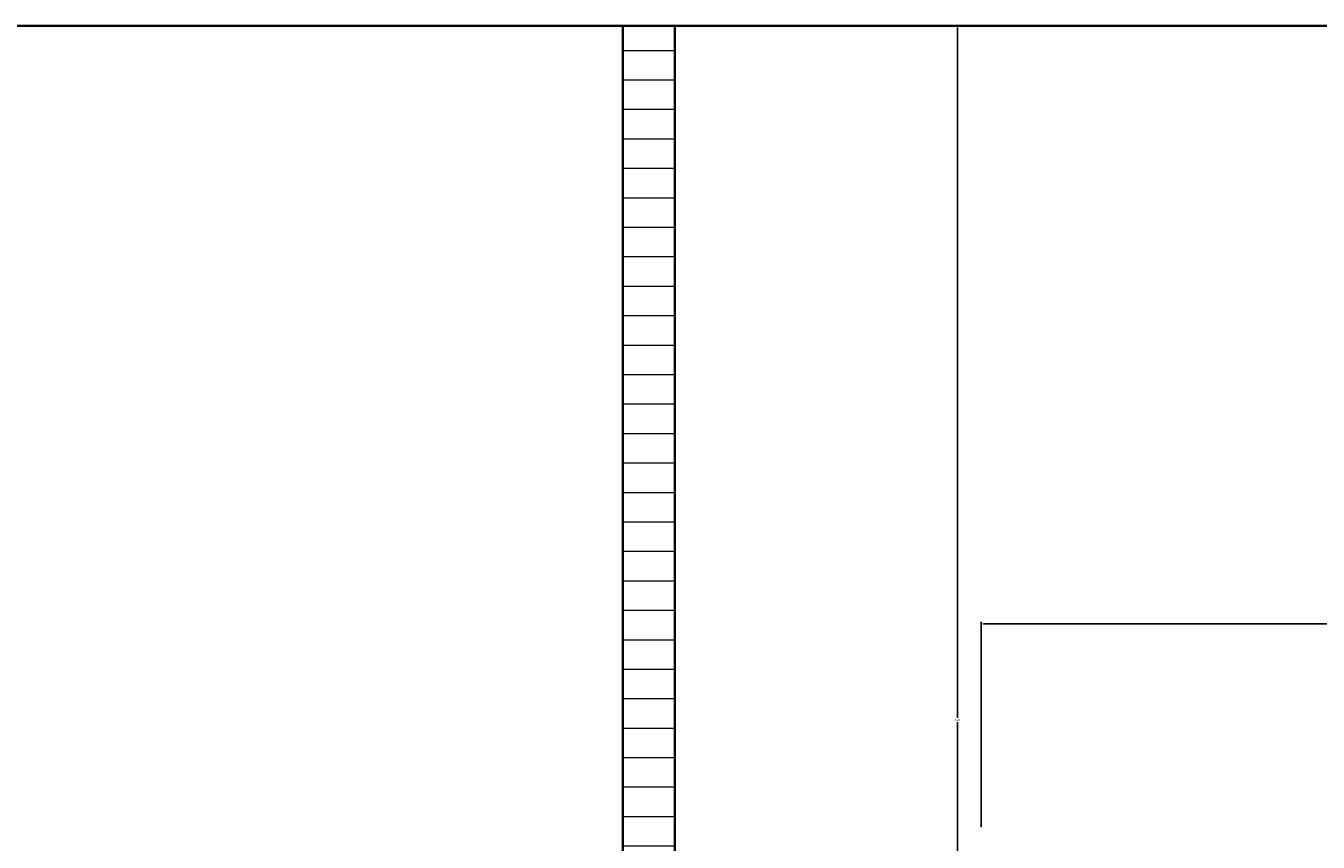
# Model space of a CAD drawing. Units: inches. Extents: x 2416 to 3391, y 1375 to 2496.
# Tile 10 of 13: x 2994 to 3105, y 2193 to 2264. Entities that reach past the tile are written whole.
import ezdxf

# ---------------------------------------------------------------- set-up
doc = ezdxf.new("R2010")
doc.units = ezdxf.units.IN
for name, color, linetype, lineweight in [('A-ANNO-DIMS', 2, 'Continuous', 18), ('A-SECT', 7, 'Continuous', 35), ('A-WALL-PATT', 252, 'Continuous', 13)]:
    doc.layers.add(name, color=color, linetype=linetype, lineweight=lineweight)
doc.styles.get("Standard").update_dxf_attribs({"font": 'arial.ttf'})
doc.dimstyles.get("Standard").update_dxf_attribs({"dimtxt": 0.18, "dimasz": 0.18, "dimexe": 0.18, "dimexo": 0.0625, "dimgap": 0.09, "dimtad": 0, "dimtih": 1, "dimtoh": 1, "dimdec": 4, "dimzin": 0, "dimdsep": 46, "dimtxsty": 'Standard', "dimcen": 0.09, "dimadec": 0, "dimazin": 0, "dimtfac": 1, "dimtdec": 4, "dimtofl": 0, "dimtmove": 0, "dimatfit": 3, "dimfxl": 1, "dimtolj": 1, "dimtzin": 0, "dimarcsym": 0})

# ---------------------------------------------------------------- blocks, each defined once
blk = doc.blocks.new('*D45')
at = {"layer": 'A-ANNO-DIMS', "color": 0, "lineweight": -2, "transparency": 16777216}
for p, q in [((3076.16, 2194.58), (3076.16, 2212.34)), ((3076.34, 2212.16), (3133.82, 2212.16)), ((3193.6, 2212.16), (3136.12, 2212.16)), ((3193.78, 2194.58), (3193.78, 2212.34))]:
    blk.add_line(p, q, dxfattribs=at)
at = {"layer": 'A-ANNO-DIMS', "color": 0, "transparency": 16777216}
for points in [[(3076.34, 2212.19), (3076.34, 2212.13), (3076.16, 2212.16)], [(3193.6, 2212.19), (3193.6, 2212.13), (3193.78, 2212.16)]]:
    blk.add_solid(points, dxfattribs=at)
at = {"layer": 'Defpoints', "color": 0, "transparency": 16777216}
for p in [(3076.16, 2212.16), (3076.16, 2194.51), (3193.78, 2194.51)]:
    blk.add_point(p, dxfattribs=at)
at = {"layer": 'A-ANNO-DIMS', "color": 0, "transparency": 16777216, "insert": (3134.97, 2212.16), "char_height": 0.18, "attachment_point": 5}
blk.add_mtext('\\A1;BED PROFILE 118', dxfattribs=at)
blk = doc.blocks.new('*D86')
at = {"layer": 'A-ANNO-DIMS', "color": 0, "lineweight": -2, "transparency": 16777216}
for p, q in [((3049.75, 2263.86), (3074.27, 2263.86)), ((3074.09, 2263.68), (3074.09, 2204.04)), ((3074.09, 2144.04), (3074.09, 2203.68)), ((3049.75, 2143.86), (3074.27, 2143.86))]:
    blk.add_line(p, q, dxfattribs=at)
at = {"layer": 'A-ANNO-DIMS', "color": 0, "transparency": 16777216}
for points in [[(3074.06, 2263.68), (3074.12, 2263.68), (3074.09, 2263.86)], [(3074.06, 2144.04), (3074.12, 2144.04), (3074.09, 2143.86)]]:
    blk.add_solid(points, dxfattribs=at)
at = {"layer": 'Defpoints', "color": 0, "transparency": 16777216}
for p in [(3049.69, 2263.86), (3049.69, 2143.86), (3074.09, 2143.86)]:
    blk.add_point(p, dxfattribs=at)
at = {"layer": 'A-ANNO-DIMS', "color": 0, "transparency": 16777216, "insert": (3074.09, 2203.86), "char_height": 0.18, "attachment_point": 5}
blk.add_mtext('\\A1;120', dxfattribs=at)

msp = doc.modelspace()

# ---------------------------------------------------------------- hatches: boundary and pattern name
at = {"layer": 'A-WALL-PATT'}
h = msp.add_hatch(dxfattribs=at)
h.set_pattern_fill('ANSI31', color=256, scale=0.802205, angle=-45, style=0)
h.paths.add_polyline_path([(3045.1924, 2143.8608), (3049.6924, 2143.8608), (3049.6924, 2263.8608), (3045.1924, 2263.8608)])

# ---------------------------------------------------------------- linework, layer by layer
at = {"layer": 'A-SECT'}
for p, q in [((3202.6924, 2263.8608), (2904.1924, 2263.8608)), ((3045.1924, 2263.8608), (3045.1924, 2143.8608)), ((3049.6924, 2263.8608), (3049.6924, 2143.8608))]:
    msp.add_line(p, q, dxfattribs=at)

# ---------------------------------------------------------------- dimensions: what is measured, and where the dimension line sits
at = {"layer": 'A-ANNO-DIMS'}
dim = msp.add_linear_dim(base=(3074.0924, 2143.8608), p1=(3049.6924, 2263.8608), p2=(3049.6924, 2143.8608), angle=270, dimstyle='Standard', override={"dimdec": 0, "dimlfac": 1, "dimrnd": 0, "dimzin": 0, "dimdsep": 46, "dimlunit": 2}, dxfattribs=at)
dim.commit()
dim.dimension.update_dxf_attribs({"geometry": '*D86', "text_midpoint": (3074.0924, 2203.8608)})
dim = msp.add_linear_dim(base=(3076.1636, 2212.1562), p1=(3193.7816, 2194.5135), p2=(3076.1636, 2194.5135), angle=180, text='BED PROFILE <>', dimstyle='Standard', override={"dimdec": 0, "dimlfac": 1, "dimrnd": 0, "dimzin": 0, "dimdsep": 46, "dimlunit": 2}, dxfattribs=at)
dim.commit()
dim.dimension.update_dxf_attribs({"geometry": '*D45', "text_midpoint": (3134.9726, 2212.1562)})

doc.saveas('drawing.dxf')
